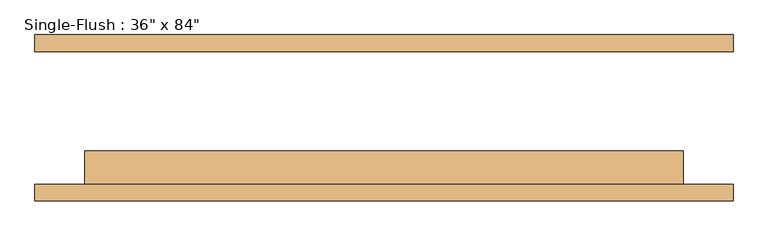
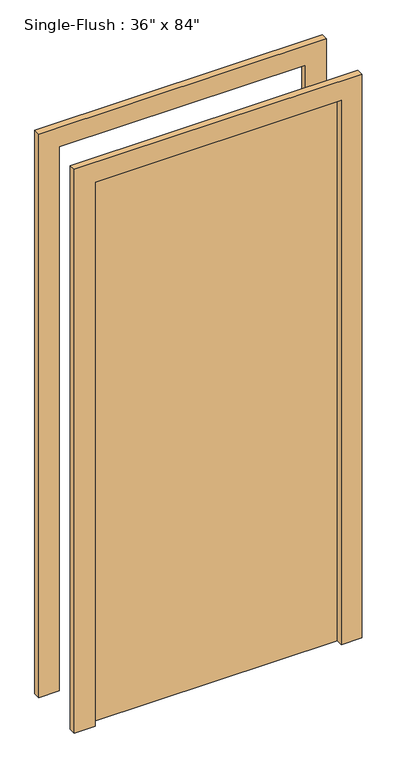
"""IFC4 building model written with IfcOpenShell, lengths in millimetres: door geometry."""

from ifc_helpers import new_model, si_unit, frame, origin, origin_with_axes, place, context, project, spatial, polyline, outline, extrude, source, transform, mapped, element, save


def door_719f80de(model_context):
    return source(origin(), model_context, "Body", "SweptSolid", [
        extrude(outline(polyline([(2209.8, -533.4), (0.0, -533.4), (0.0, -457.2), (2133.6, -457.2), (2133.6, 457.2), (0.0, 457.2), (0.0, 533.4), (2209.8, 533.4), (2209.8, -533.4)])), frame((0.0, -127.0, 0.0), z_axis=(0.0, 1.0, 0.0), x_axis=(0.0, 0.0, 1.0)), (0.0, 0.0, 1.0), 25.4),
        extrude(outline(polyline([(2209.8, 533.4), (2209.8, -533.4), (0.0, -533.4), (0.0, -457.2), (2133.6, -457.2), (2133.6, 457.2), (0.0, 457.2), (0.0, 533.4), (2209.8, 533.4)])), frame((0.0, 101.6, 0.0), z_axis=(0.0, 1.0, 0.0), x_axis=(0.0, 0.0, 1.0)), (0.0, 0.0, 1.0), 25.4),
        extrude(outline(polyline([(457.2, -50.8), (457.2, -101.6), (-457.2, -101.6), (-457.2, -50.8), (457.2, -50.8)])), origin_with_axes(), (0.0, 0.0, 1.0), 2133.6),
    ])


if __name__ == "__main__":
    model = new_model("IFC4")
    model_context = context("Model", 3, world=origin())
    ifc_project = project(units=[si_unit("LENGTHUNIT", "METRE", prefix="MILLI")], contexts=[model_context])
    site = spatial("IfcSite", under=ifc_project)
    building = spatial("IfcBuilding", under=site)
    placement = place(None, origin())
    door_shape = door_719f80de(model_context)
    element("IfcDoor", 1, ObjectType="Single-Flush : 36\" x 84\"", at=placement, inside=building, context=model_context, shape_type="MappedRepresentation", body=[
        mapped(door_shape, transform((0.0, 0.0, 0.0), x_axis=(1.0, 0.0, 0.0), y_axis=(0.0, 1.0, 0.0), z_axis=(0.0, 0.0, 1.0))),
    ])
    save(model, "model.ifc")

# Revit data of these elements
# Type "Single-Flush : 36\" x 84\""
#   Type Mark = "1"
#   Construction Type Id = "MDOOR"
#   Assembly Code = "C1020"
#   Analytic Construction = "Metal"
#   Thickness = 0' - 2"
#   Heat Transfer Coefficient (U) = 0.651978 BTU/(h·ft²·°F)
#   Height = 7' - 0"
#   Trim Projection Ext = 0' - 1"
#   Trim Projection Int = 0' - 1"
#   Trim Width = 0' - 3"
#   Width = 3' - 0"
#   Define Thermal Properties by = 1
#   Define Thermal Properties by = 1
#   Door Material = Door - Panel
#   Frame Material = Door - Frame
#   Visual Light Transmittance = 0
#   Solar Heat Gain Coefficient = 0
#   Function = (empty or 0)
#   Wall Closure = (empty or 0)
# Element 1 (IfcDoor, "Single-Flush : 36\" x 84\"")
#   Materials on its faces: "Door - Frame", "Door - Panel"
# Materials
#   "Door - Panel": class "Wood", colour RGB 210 159 95, transparency 0, Cost = 0
#   "Door - Frame": colour RGB 118 70 51, transparency 0, Cost = 0
